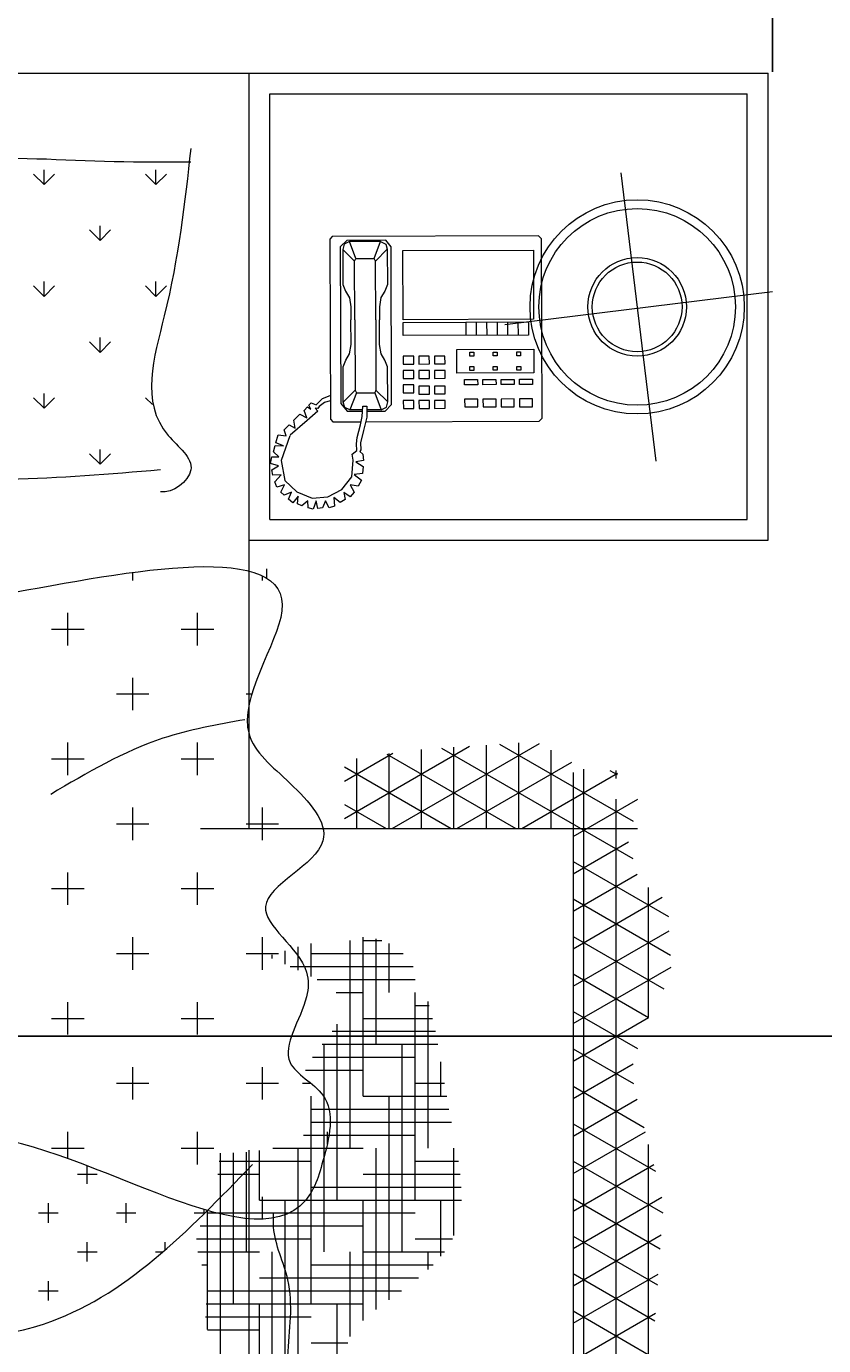
# Model space of a CAD drawing. Units: inches. Extents: x 2330 to 3943, y 1763 to 3461.
# Tile 7 of 40: x 2593 to 2634, y 2316 to 2383. Entities that reach past the tile are written whole.
import ezdxf

# ---------------------------------------------------------------- set-up
doc = ezdxf.new("R2010")
doc.units = ezdxf.units.IN
doc.layers.add('A-ANNO-DIMS', color=2, linetype='Continuous', lineweight=18)
doc.layers.add('A-FURN', color=8, linetype='Continuous', lineweight=13)
doc.styles.get("Standard").update_dxf_attribs({"font": 'arial.ttf'})
doc.dimstyles.get("Standard").update_dxf_attribs({"dimtxt": 0.18, "dimasz": 0.18, "dimexe": 0.18, "dimexo": 0.0625, "dimgap": 0.09, "dimtad": 0, "dimtih": 1, "dimtoh": 1, "dimdec": 4, "dimzin": 0, "dimdsep": 46, "dimtxsty": 'Standard', "dimcen": 0.09, "dimadec": 0, "dimazin": 0, "dimtfac": 1, "dimtdec": 4, "dimtofl": 0, "dimtmove": 0, "dimatfit": 3, "dimfxl": 1, "dimtolj": 1, "dimtzin": 0, "dimarcsym": 0})

# ---------------------------------------------------------------- blocks, each defined once
blk = doc.blocks.new('A$C200C7901')
for p, q in [((0.5, 2.3334), (2, 2.3334)), ((2, 2.3334), (2.5, 2.3334)), ((2, 1.6055), (2, 2.3334)), ((2.5, 1.8834), (2.5, 2.3334)), ((2, 1.8834), (2.5, 1.8834)), ((2.0171, 1.8467), (2.0171, 1.8556)), ((2.0171, 1.8467), (2.0171, 1.8556)), ((2.0129, 1.8445), (2.0129, 1.849)), ((2.0129, 1.8445), (2.0129, 1.849)), ((1.9972, 1.7352), (2.0027, 1.7352)), ((1.9972, 1.7352), (2.0027, 1.7352)), ((2, 1.6963), (2, 1.7248)), ((2, 1.6963), (2, 1.7248)), ((2.3121, 1.6596), (2.3121, 0.0201)), ((1.9533, 1.6055), (2.3741, 1.6055)), ((1.9533, 1.6055), (2.3741, 1.6055)), ((2, 0.2957), (2, 1.2957)), ((2.0224, 0.9977), (2.0224, 1.1977)), ((2.0224, 0.9977), (2.0224, 1.1977))]:
    blk.add_line(p, q)
at = {"linetype": 'ByBlock'}
for p, q in [((2.02, 2.3134), (2.48, 2.3134)), ((2.02, 1.9034), (2.02, 2.3134)), ((2.48, 1.9034), (2.48, 2.3134)), ((1.8025, 2.2259), (1.8025, 2.2402)), ((1.8025, 2.2259), (1.8025, 2.2402)), ((1.9103, 2.2259), (1.9103, 2.2402)), ((1.9103, 2.2259), (1.9103, 2.2402)), ((2.3581, 2.2373), (2.3919, 1.9595)), ((1.8025, 2.2259), (1.7924, 2.236)), ((1.8025, 2.2259), (1.7924, 2.236)), ((1.8025, 2.2259), (1.8126, 2.236)), ((1.8025, 2.2259), (1.8126, 2.236)), ((1.9103, 2.2259), (1.9002, 2.236)), ((1.9103, 2.2259), (1.9002, 2.236)), ((1.9103, 2.2259), (1.9204, 2.236)), ((1.9103, 2.2259), (1.9204, 2.236)), ((1.8564, 2.172), (1.8564, 2.1863)), ((1.8564, 2.172), (1.8564, 2.1863)), ((1.8564, 2.1721), (1.8463, 2.1822)), ((1.8564, 2.1721), (1.8463, 2.1822)), ((1.8564, 2.1721), (1.8665, 2.1822)), ((1.8564, 2.1721), (1.8665, 2.1822)), ((2.0802, 2.176), (2.0777, 2.1734)), ((2.0777, 2.1734), (2.0783, 1.9999)), ((2.2789, 2.1766), (2.0802, 2.176)), ((2.2789, 2.1766), (2.2814, 2.1741)), ((2.2814, 2.1741), (2.282, 2.0006)), ((2.0941, 2.1722), (2.0878, 2.1659)), ((2.0878, 2.1659), (2.0883, 2.015)), ((2.0915, 2.1685), (2.0903, 2.1634)), ((2.0903, 2.1634), (2.1017, 2.1521)), ((2.0903, 2.1634), (2.0904, 2.1295)), ((2.0966, 2.171), (2.0915, 2.1685)), ((2.1318, 2.1724), (2.0941, 2.1722)), ((2.1267, 2.1711), (2.0966, 2.171)), ((2.1029, 2.1547), (2.0966, 2.171)), ((2.1205, 2.1547), (2.1267, 2.1711)), ((2.1331, 2.1636), (2.1218, 2.1522)), ((2.1267, 2.1711), (2.1318, 2.1686)), ((2.1368, 2.1661), (2.1318, 2.1724)), ((2.1318, 2.1686), (2.1331, 2.1636)), ((2.1331, 2.1636), (2.1332, 2.1296)), ((2.1373, 2.014), (2.1368, 2.1661)), ((2.1481, 2.1624), (2.2739, 2.1628)), ((2.1484, 2.0957), (2.1481, 2.1624)), ((2.2739, 2.1628), (2.2741, 2.0961)), ((2.1017, 2.1521), (2.1029, 2.1547)), ((2.1019, 2.0956), (2.1017, 2.1521)), ((2.1029, 2.1547), (2.1205, 2.1547)), ((2.1218, 2.1522), (2.1205, 2.1547)), ((2.122, 2.0956), (2.1218, 2.1522)), ((1.8025, 2.1182), (1.7924, 2.1283)), ((1.8025, 2.1182), (1.7924, 2.1283)), ((1.8025, 2.1182), (1.8025, 2.1325)), ((1.8025, 2.1182), (1.8025, 2.1325)), ((1.8025, 2.1182), (1.8126, 2.1283)), ((1.8025, 2.1182), (1.8126, 2.1283)), ((1.9103, 2.1182), (1.9002, 2.1283)), ((1.9103, 2.1182), (1.9002, 2.1283)), ((1.9103, 2.1182), (1.9103, 2.1325)), ((1.9103, 2.1182), (1.9103, 2.1325)), ((1.9103, 2.1182), (1.9204, 2.1283)), ((1.9103, 2.1182), (1.9204, 2.1283)), ((2.0904, 2.1295), (2.093, 2.1232)), ((2.093, 2.1232), (2.0968, 2.1169)), ((2.1307, 2.1233), (2.1269, 2.117)), ((2.1332, 2.1296), (2.1307, 2.1233)), ((2.2464, 2.0911), (2.5044, 2.1228)), ((2.0968, 2.1169), (2.098, 2.1081)), ((2.1269, 2.117), (2.1257, 2.1082)), ((2.098, 2.1081), (2.0981, 2.0956)), ((2.1257, 2.1082), (2.1257, 2.0956)), ((2.0982, 2.0717), (2.0981, 2.0956)), ((2.1019, 2.0956), (2.1021, 2.0277)), ((2.122, 2.0956), (2.1222, 2.0277)), ((2.1258, 2.0718), (2.1257, 2.0956)), ((2.2741, 2.0961), (2.1484, 2.0957)), ((2.1484, 2.0932), (2.2691, 2.0936)), ((2.1484, 2.0806), (2.1484, 2.0932)), ((2.2087, 2.0934), (2.2088, 2.0808)), ((2.2188, 2.0934), (2.2188, 2.0809)), ((2.2288, 2.0935), (2.2289, 2.0809)), ((2.2389, 2.0935), (2.239, 2.0809)), ((2.249, 2.0935), (2.249, 2.081)), ((2.259, 2.0936), (2.2591, 2.081)), ((2.2691, 2.0936), (2.2691, 2.081)), ((1.8564, 2.0643), (1.8463, 2.0744)), ((1.8564, 2.0643), (1.8463, 2.0744)), ((1.8564, 2.0643), (1.8564, 2.0786)), ((1.8564, 2.0643), (1.8564, 2.0786)), ((1.8564, 2.0643), (1.8665, 2.0744)), ((1.8564, 2.0643), (1.8665, 2.0744)), ((2.0969, 2.0629), (2.0982, 2.0717)), ((2.1271, 2.063), (2.1258, 2.0718)), ((2.2691, 2.081), (2.1484, 2.0806)), ((2.0932, 2.0566), (2.0969, 2.0629)), ((2.1309, 2.0567), (2.1271, 2.063)), ((2.1586, 2.0606), (2.1485, 2.0605)), ((2.1485, 2.0605), (2.1485, 2.053)), ((2.1586, 2.053), (2.1586, 2.0606)), ((2.1636, 2.0606), (2.1636, 2.053)), ((2.1736, 2.0606), (2.1636, 2.0606)), ((2.1737, 2.0531), (2.1736, 2.0606)), ((2.1887, 2.0607), (2.1787, 2.0606)), ((2.1787, 2.0606), (2.1787, 2.0531)), ((2.1888, 2.0531), (2.1887, 2.0607)), ((2.2, 2.067), (2.2742, 2.0672)), ((2.2001, 2.0443), (2.2, 2.067)), ((2.2126, 2.0645), (2.2164, 2.0645)), ((2.2126, 2.0607), (2.2126, 2.0645)), ((2.2164, 2.0607), (2.2126, 2.0607)), ((2.2164, 2.0645), (2.2164, 2.0607)), ((2.2352, 2.0646), (2.239, 2.0646)), ((2.2352, 2.0608), (2.2352, 2.0646)), ((2.239, 2.0608), (2.2352, 2.0608)), ((2.239, 2.0646), (2.239, 2.0608)), ((2.2579, 2.0609), (2.2579, 2.0647)), ((2.2579, 2.0647), (2.2616, 2.0647)), ((2.2616, 2.0609), (2.2579, 2.0609)), ((2.2616, 2.0647), (2.2616, 2.0609)), ((2.2742, 2.0672), (2.2743, 2.0446)), ((2.0907, 2.0503), (2.0932, 2.0566)), ((2.0908, 2.0163), (2.0907, 2.0503)), ((2.1334, 2.0504), (2.1309, 2.0567)), ((2.1336, 2.0165), (2.1334, 2.0504)), ((2.1485, 2.053), (2.1586, 2.053)), ((2.1485, 2.0467), (2.1486, 2.0391)), ((2.1586, 2.0467), (2.1485, 2.0467)), ((2.1586, 2.0392), (2.1586, 2.0467)), ((2.1636, 2.053), (2.1737, 2.0531)), ((2.1737, 2.0468), (2.1636, 2.0467)), ((2.1636, 2.0467), (2.1637, 2.0392)), ((2.1737, 2.0392), (2.1737, 2.0468)), ((2.1787, 2.0531), (2.1888, 2.0531)), ((2.1787, 2.0468), (2.1787, 2.0392)), ((2.1888, 2.0468), (2.1787, 2.0468)), ((2.1888, 2.0393), (2.1888, 2.0468)), ((2.2126, 2.0507), (2.2164, 2.0507)), ((2.2127, 2.0469), (2.2126, 2.0507)), ((2.2164, 2.0469), (2.2127, 2.0469)), ((2.2164, 2.0507), (2.2164, 2.0469)), ((2.2353, 2.0508), (2.2391, 2.0508)), ((2.2353, 2.047), (2.2353, 2.0508)), ((2.2391, 2.047), (2.2353, 2.047)), ((2.2391, 2.0508), (2.2391, 2.047)), ((2.2579, 2.0508), (2.2617, 2.0508)), ((2.2579, 2.0471), (2.2579, 2.0508)), ((2.2617, 2.0471), (2.2579, 2.0471)), ((2.2617, 2.0508), (2.2617, 2.0471)), ((2.1486, 2.0391), (2.1586, 2.0392)), ((2.1637, 2.0392), (2.1737, 2.0392)), ((2.1787, 2.0392), (2.1888, 2.0393)), ((2.2743, 2.0446), (2.2001, 2.0443)), ((2.2077, 2.0331), (2.2077, 2.0381)), ((2.2077, 2.0381), (2.2202, 2.0381)), ((2.2202, 2.0381), (2.2203, 2.0331)), ((2.2253, 2.0381), (2.2378, 2.0382)), ((2.2253, 2.0331), (2.2253, 2.0381)), ((2.2378, 2.0382), (2.2379, 2.0332)), ((2.2429, 2.0332), (2.2429, 2.0382)), ((2.2429, 2.0382), (2.2554, 2.0382)), ((2.2554, 2.0382), (2.2555, 2.0332)), ((2.2605, 2.0332), (2.2605, 2.0383)), ((2.2605, 2.0383), (2.273, 2.0383)), ((2.273, 2.0383), (2.2731, 2.0333)), ((1.8025, 2.0104), (1.8025, 2.0247)), ((1.8025, 2.0104), (1.8025, 2.0247)), ((2.0707, 2.0197), (2.0782, 2.0226)), ((2.0908, 2.0163), (2.1021, 2.0277)), ((2.1034, 2.0252), (2.0971, 2.0088)), ((2.1021, 2.0277), (2.1034, 2.0252)), ((2.1034, 2.0252), (2.121, 2.0252)), ((2.1222, 2.0277), (2.121, 2.0252)), ((2.121, 2.0252), (2.1273, 2.0089)), ((2.1336, 2.0165), (2.1222, 2.0277)), ((2.1586, 2.0329), (2.1486, 2.0329)), ((2.1486, 2.0329), (2.1486, 2.0253)), ((2.1486, 2.0253), (2.1587, 2.0253)), ((2.1587, 2.0253), (2.1586, 2.0329)), ((2.1637, 2.0317), (2.1637, 2.0241)), ((2.1737, 2.0317), (2.1637, 2.0317)), ((2.1637, 2.0241), (2.1738, 2.0241)), ((2.1738, 2.0241), (2.1737, 2.0317)), ((2.1788, 2.0317), (2.1788, 2.0242)), ((2.1888, 2.0317), (2.1788, 2.0317)), ((2.1788, 2.0242), (2.1889, 2.0242)), ((2.1889, 2.0242), (2.1888, 2.0317)), ((2.2203, 2.0331), (2.2077, 2.0331)), ((2.2379, 2.0332), (2.2253, 2.0331)), ((2.2555, 2.0332), (2.2429, 2.0332)), ((2.2731, 2.0333), (2.2605, 2.0332)), ((1.8025, 2.0104), (1.7924, 2.0205)), ((1.8025, 2.0104), (1.7924, 2.0205)), ((1.8025, 2.0104), (1.8126, 2.0205)), ((1.8025, 2.0104), (1.8126, 2.0205)), ((1.9068, 2.0139), (1.9002, 2.0205)), ((1.9068, 2.0139), (1.9002, 2.0205)), ((2.053, 2.0084), (2.0563, 2.0119)), ((2.0557, 2.0011), (2.053, 2.0084)), ((2.0563, 2.0119), (2.0594, 2.0095)), ((2.0576, 2.0133), (2.0598, 2.0155)), ((2.0594, 2.0095), (2.0576, 2.0133)), ((2.0598, 2.0155), (2.0645, 2.0137)), ((2.0663, 2.0102), (2.0636, 2.0104)), ((2.0636, 2.0104), (2.0663, 2.0077)), ((2.0645, 2.0137), (2.0671, 2.0162)), ((2.0676, 2.012), (2.0663, 2.0102)), ((2.0671, 2.0162), (2.0707, 2.0197)), ((2.0727, 2.016), (2.0676, 2.012)), ((2.0782, 2.0175), (2.0727, 2.016)), ((2.0883, 2.015), (2.0946, 2.0075)), ((2.0921, 2.0113), (2.0908, 2.0163)), ((2.0971, 2.0088), (2.0921, 2.0113)), ((2.1094, 2.0088), (2.0971, 2.0088)), ((2.109, 2.0025), (2.1097, 2.0126)), ((2.1097, 2.0126), (2.1135, 2.0126)), ((2.1135, 2.0126), (2.1133, 2.0018)), ((2.1273, 2.0089), (2.1134, 2.0088)), ((2.1273, 2.0089), (2.1323, 2.0114)), ((2.1311, 2.0077), (2.1373, 2.014)), ((2.1323, 2.0114), (2.1336, 2.0165)), ((2.1587, 2.0178), (2.1486, 2.0178)), ((2.1486, 2.0178), (2.1487, 2.0102)), ((2.1487, 2.0102), (2.1587, 2.0103)), ((2.1587, 2.0103), (2.1587, 2.0178)), ((2.1738, 2.0179), (2.1637, 2.0178)), ((2.1637, 2.0178), (2.1638, 2.0103)), ((2.1638, 2.0103), (2.1738, 2.0103)), ((2.1738, 2.0103), (2.1738, 2.0179)), ((2.1788, 2.0179), (2.1788, 2.0103)), ((2.1889, 2.0179), (2.1788, 2.0179)), ((2.1788, 2.0103), (2.1889, 2.0104)), ((2.1889, 2.0104), (2.1889, 2.0179)), ((2.2203, 2.0193), (2.2077, 2.0192)), ((2.2077, 2.0192), (2.2078, 2.0117)), ((2.2078, 2.0117), (2.2203, 2.0117)), ((2.2203, 2.0117), (2.2203, 2.0193)), ((2.2379, 2.0193), (2.2253, 2.0193)), ((2.2253, 2.0193), (2.2254, 2.0117)), ((2.2254, 2.0117), (2.2379, 2.0118)), ((2.2379, 2.0118), (2.2379, 2.0193)), ((2.2555, 2.0194), (2.2429, 2.0193)), ((2.2429, 2.0193), (2.243, 2.0118)), ((2.243, 2.0118), (2.2555, 2.0118)), ((2.2555, 2.0118), (2.2555, 2.0194)), ((2.2605, 2.0194), (2.2606, 2.0119)), ((2.2731, 2.0194), (2.2605, 2.0194)), ((2.2606, 2.0119), (2.2731, 2.0119)), ((2.2731, 2.0119), (2.2731, 2.0194)), ((2.0561, 1.9986), (2.0396, 1.9844)), ((2.0431, 1.999), (2.0488, 2.0046)), ((2.0444, 1.9911), (2.0431, 1.999)), ((2.0488, 2.0046), (2.0557, 2.0011)), ((2.0663, 2.0077), (2.0561, 1.9986)), ((2.0783, 1.9999), (2.0808, 1.9974)), ((2.0808, 1.9974), (2.1079, 1.9975)), ((2.0946, 2.0075), (2.1093, 2.0076)), ((2.1072, 1.9944), (2.109, 2.0025)), ((2.1133, 2.0018), (2.1103, 1.989)), ((2.1123, 1.9975), (2.2795, 1.9981)), ((2.1134, 2.0076), (2.1311, 2.0077)), ((2.282, 2.0006), (2.2795, 1.9981)), ((2.0259, 1.977), (2.0281, 1.9847)), ((2.0281, 1.9847), (2.0358, 1.9839)), ((2.0393, 1.984), (2.031, 1.96)), ((2.0338, 1.9895), (2.0386, 1.9946)), ((2.0358, 1.9839), (2.0338, 1.9895)), ((2.0386, 1.9946), (2.0444, 1.9911)), ((2.1042, 1.9824), (2.1072, 1.9944)), ((2.1103, 1.989), (2.1073, 1.9771)), ((1.8564, 1.9565), (1.8564, 1.9708)), ((1.8564, 1.9565), (1.8564, 1.9708)), ((2.0234, 1.9686), (2.0251, 1.9745)), ((2.0251, 1.9745), (2.0333, 1.9743)), ((2.0333, 1.9743), (2.0259, 1.977)), ((2.1035, 1.9763), (2.1042, 1.9824)), ((2.1038, 1.9697), (2.1035, 1.9763)), ((2.1076, 1.9704), (2.1068, 1.9689)), ((2.1073, 1.9771), (2.1076, 1.9704)), ((1.8564, 1.9565), (1.8463, 1.9666)), ((1.8564, 1.9565), (1.8463, 1.9666)), ((1.8564, 1.9565), (1.8665, 1.9666)), ((1.8564, 1.9565), (1.8665, 1.9666)), ((2.0206, 1.9572), (2.0218, 1.9635)), ((2.0285, 1.9549), (2.0206, 1.9572)), ((2.0218, 1.9635), (2.0287, 1.9636)), ((2.0287, 1.9636), (2.0234, 1.9686)), ((2.031, 1.96), (2.0346, 1.9409)), ((2.099, 1.9444), (2.1002, 1.9605)), ((2.0992, 1.9663), (2.1038, 1.9697)), ((2.1002, 1.9605), (2.0992, 1.9663)), ((2.1101, 1.96), (2.1028, 1.9587)), ((2.1028, 1.9587), (2.1099, 1.9544)), ((2.1068, 1.9689), (2.1096, 1.9661)), ((2.1096, 1.9661), (2.1101, 1.96)), ((2.0219, 1.9511), (2.0285, 1.9549)), ((2.0229, 1.946), (2.0219, 1.9511)), ((2.0308, 1.9462), (2.0229, 1.946)), ((2.0247, 1.9394), (2.0308, 1.9462)), ((2.1094, 1.9475), (2.1013, 1.9467)), ((2.1013, 1.9467), (2.1084, 1.9412)), ((2.1099, 1.9544), (2.1094, 1.9475)), ((2.0268, 1.9343), (2.0247, 1.9394)), ((2.0341, 1.9366), (2.0268, 1.9343)), ((2.0306, 1.9297), (2.0341, 1.9366)), ((2.0346, 1.9409), (2.0459, 1.93)), ((2.0759, 1.925), (2.0894, 1.9322)), ((2.0894, 1.9322), (2.099, 1.9444)), ((2.1051, 1.9353), (2.0975, 1.9368)), ((2.0975, 1.9368), (2.1011, 1.9297)), ((2.1084, 1.9412), (2.1051, 1.9353)), ((2.0339, 1.9267), (2.0306, 1.9297)), ((2.041, 1.9297), (2.0339, 1.9267)), ((2.038, 1.9228), (2.041, 1.9297)), ((2.0421, 1.9193), (2.038, 1.9228)), ((2.0474, 1.9259), (2.0421, 1.9193)), ((2.0459, 1.93), (2.0607, 1.9237)), ((2.0467, 1.9183), (2.0474, 1.9259)), ((2.0566, 1.9214), (2.0508, 1.9163)), ((2.0569, 1.9145), (2.0566, 1.9214)), ((2.0607, 1.9237), (2.0759, 1.925)), ((2.0645, 1.9214), (2.0617, 1.9133)), ((2.0663, 1.914), (2.0645, 1.9214)), ((2.0736, 1.9214), (2.0706, 1.9146)), ((2.077, 1.9146), (2.0736, 1.9214)), ((2.0876, 1.9195), (2.0815, 1.9245)), ((2.0815, 1.9245), (2.0823, 1.9161)), ((2.0925, 1.9225), (2.0876, 1.9195)), ((2.0973, 1.9251), (2.0914, 1.9294)), ((2.0914, 1.9294), (2.0925, 1.9225)), ((2.1011, 1.9297), (2.0973, 1.9251)), ((2.0508, 1.9163), (2.0467, 1.9183)), ((2.0617, 1.9133), (2.0569, 1.9145)), ((2.0706, 1.9146), (2.0663, 1.914)), ((2.0823, 1.9161), (2.077, 1.9146)), ((2.02, 1.9034), (2.48, 1.9034)), ((1.8879, 1.8445), (1.8879, 1.8523)), ((1.8879, 1.8445), (1.8879, 1.8523)), ((1.8254, 1.782), (1.8254, 1.8133)), ((1.8254, 1.782), (1.8254, 1.8133)), ((1.9504, 1.782), (1.9504, 1.8133)), ((1.9504, 1.782), (1.9504, 1.8133)), ((1.8097, 1.7977), (1.841, 1.7977)), ((1.8097, 1.7977), (1.841, 1.7977)), ((1.9347, 1.7977), (1.966, 1.7977)), ((1.9347, 1.7977), (1.966, 1.7977)), ((1.8879, 1.7195), (1.8879, 1.7508)), ((1.8879, 1.7195), (1.8879, 1.7508)), ((1.8722, 1.7352), (1.9035, 1.7352)), ((1.8722, 1.7352), (1.9035, 1.7352)), ((1.8254, 1.657), (1.8254, 1.6883)), ((1.8254, 1.657), (1.8254, 1.6883)), ((1.9504, 1.657), (1.9504, 1.6883)), ((1.9504, 1.657), (1.9504, 1.6883)), ((2.0919, 1.6152), (2.2125, 1.6848)), ((2.0919, 1.6152), (2.2125, 1.6848)), ((2.0919, 1.6513), (2.1386, 1.6782)), ((2.0919, 1.6513), (2.1386, 1.6782)), ((2.1349, 1.6055), (2.1349, 1.6777)), ((2.1349, 1.6055), (2.1349, 1.6777)), ((2.1377, 1.6055), (2.2798, 1.6876)), ((2.1377, 1.6055), (2.2798, 1.6876)), ((2.1662, 1.6055), (2.1662, 1.6817)), ((2.1662, 1.6055), (2.1662, 1.6817)), ((2.1854, 1.683), (2.3697, 1.5766)), ((2.1854, 1.683), (2.3697, 1.5766)), ((2.1974, 1.6055), (2.1974, 1.6838)), ((2.1974, 1.6055), (2.1974, 1.6838)), ((2.2287, 1.6055), (2.2287, 1.6859)), ((2.2287, 1.6055), (2.2287, 1.6859)), ((2.2414, 1.6868), (2.3699, 1.6126)), ((2.2414, 1.6868), (2.3699, 1.6126)), ((2.2599, 1.6055), (2.2599, 1.688)), ((2.2599, 1.6055), (2.2599, 1.688)), ((2.2912, 1.6055), (2.2912, 1.6809)), ((2.2912, 1.6055), (2.2912, 1.6809)), ((1.8097, 1.6727), (1.841, 1.6727)), ((1.8097, 1.6727), (1.841, 1.6727)), ((1.9347, 1.6727), (1.966, 1.6727)), ((1.9347, 1.6727), (1.966, 1.6727)), ((2.1037, 1.6055), (2.1037, 1.673)), ((2.1037, 1.6055), (2.1037, 1.673)), ((2.1327, 1.6773), (2.2571, 1.6055)), ((2.1327, 1.6773), (2.2571, 1.6055)), ((2.2002, 1.6055), (2.3109, 1.6694)), ((2.2002, 1.6055), (2.3109, 1.6694)), ((2.0919, 1.6649), (2.1946, 1.6055)), ((2.0919, 1.6649), (2.1946, 1.6055)), ((2.2627, 1.6055), (2.3551, 1.6589)), ((2.2627, 1.6055), (2.3551, 1.6589)), ((2.3224, 0.0468), (2.3224, 1.6627)), ((2.3224, 0.0468), (2.3224, 1.6627)), ((2.3476, 1.6616), (2.3547, 1.6575)), ((2.3476, 1.6616), (2.3547, 1.6575)), ((2.3537, 1.6539), (2.3537, 1.6616)), ((2.3537, 1.6539), (2.3537, 1.6616)), ((2.0919, 1.6288), (2.1321, 1.6055)), ((2.0919, 1.6288), (2.1321, 1.6055)), ((2.3121, 1.598), (2.3745, 1.634)), ((2.3121, 1.598), (2.3745, 1.634)), ((2.3537, 0.0056), (2.3537, 1.634)), ((2.3537, 0.0056), (2.3537, 1.634)), ((1.8879, 1.5945), (1.8879, 1.6258)), ((1.8879, 1.5945), (1.8879, 1.6258)), ((2.0129, 1.5945), (2.0129, 1.6258)), ((2.0129, 1.5945), (2.0129, 1.6258)), ((1.8722, 1.6102), (1.9035, 1.6102)), ((1.8722, 1.6102), (1.9035, 1.6102)), ((1.9972, 1.6102), (2.0285, 1.6102)), ((1.9972, 1.6102), (2.0285, 1.6102)), ((2.3121, 1.5619), (2.3654, 1.5926)), ((2.3121, 1.5619), (2.3654, 1.5926)), ((1.8254, 1.532), (1.8254, 1.5633)), ((1.8254, 1.532), (1.8254, 1.5633)), ((1.9504, 1.532), (1.9504, 1.5633)), ((1.9504, 1.532), (1.9504, 1.5633)), ((2.3121, 1.5738), (2.404, 1.5208)), ((2.3121, 1.5738), (2.404, 1.5208)), ((2.3121, 1.5258), (2.3739, 1.5615)), ((2.3121, 1.5258), (2.3739, 1.5615)), ((1.8097, 1.5477), (1.841, 1.5477)), ((1.8097, 1.5477), (1.841, 1.5477)), ((1.9347, 1.5477), (1.966, 1.5477)), ((1.9347, 1.5477), (1.966, 1.5477)), ((2.3121, 1.4897), (2.3979, 1.5393)), ((2.3121, 1.4897), (2.3979, 1.5393)), ((2.3849, 1.4236), (2.3849, 1.5486)), ((2.3849, 1.4236), (2.3849, 1.5486)), ((2.3121, 1.5377), (2.406, 1.4835)), ((2.3121, 1.5377), (2.406, 1.4835)), ((1.8879, 1.4695), (1.8879, 1.5008)), ((1.8879, 1.4695), (1.8879, 1.5008)), ((2.0129, 1.4695), (2.0129, 1.5008)), ((2.0129, 1.4695), (2.0129, 1.5008)), ((2.1099, 1.3477), (2.1099, 1.5009)), ((2.1099, 1.3477), (2.1099, 1.5009)), ((2.3121, 1.4537), (2.4047, 1.5071)), ((2.3121, 1.4537), (2.4047, 1.5071)), ((2.3121, 1.5016), (2.3997, 1.4511)), ((2.3121, 1.5016), (2.3997, 1.4511)), ((2.0349, 1.4748), (2.0349, 1.4879)), ((2.0349, 1.4748), (2.0349, 1.4879)), ((2.0474, 1.4691), (2.0474, 1.4915)), ((2.0474, 1.4691), (2.0474, 1.4915)), ((2.0599, 1.4631), (2.0599, 1.4948)), ((2.0599, 1.4631), (2.0599, 1.4948)), ((2.0974, 1.2977), (2.0974, 1.4977)), ((2.0974, 1.2977), (2.0974, 1.4977)), ((2.1099, 1.4977), (2.1279, 1.4977)), ((2.1099, 1.4977), (2.1279, 1.4977)), ((2.1224, 1.3977), (2.1224, 1.4992)), ((2.1224, 1.3977), (2.1224, 1.4992)), ((2.1349, 1.4477), (2.1349, 1.4949)), ((2.1349, 1.4477), (2.1349, 1.4949)), ((1.8722, 1.4852), (1.9035, 1.4852)), ((1.8722, 1.4852), (1.9035, 1.4852)), ((1.9972, 1.4852), (2.0285, 1.4852)), ((1.9972, 1.4852), (2.0285, 1.4852)), ((2.0224, 1.4805), (2.0224, 1.4839)), ((2.0224, 1.4805), (2.0224, 1.4839)), ((2.0599, 1.4852), (2.1484, 1.4852)), ((2.0599, 1.4852), (2.1484, 1.4852)), ((2.0397, 1.4727), (2.1581, 1.4727)), ((2.0397, 1.4727), (2.1581, 1.4727)), ((2.3121, 1.4176), (2.4067, 1.4721)), ((2.3121, 1.4176), (2.4067, 1.4721)), ((2.3121, 1.4655), (2.3849, 1.4235)), ((2.3121, 1.4655), (2.3849, 1.4235)), ((2.0656, 1.4602), (2.1599, 1.4602)), ((2.0656, 1.4602), (2.1599, 1.4602)), ((1.8254, 1.407), (1.8254, 1.4383)), ((1.8254, 1.407), (1.8254, 1.4383)), ((1.9504, 1.407), (1.9504, 1.4383)), ((1.9504, 1.407), (1.9504, 1.4383)), ((2.084, 1.4477), (2.1099, 1.4477)), ((2.084, 1.4477), (2.1099, 1.4477)), ((2.0849, 1.4468), (2.0849, 1.4477)), ((2.0849, 1.4468), (2.0849, 1.4477)), ((2.1599, 1.2477), (2.1599, 1.4477)), ((2.1599, 1.2477), (2.1599, 1.4477)), ((2.1724, 1.2977), (2.1724, 1.439)), ((2.1724, 1.2977), (2.1724, 1.439)), ((2.1599, 1.4352), (2.1735, 1.4352)), ((2.1599, 1.4352), (2.1735, 1.4352)), ((2.3121, 1.4294), (2.3741, 1.3937)), ((2.3121, 1.4294), (2.3741, 1.3937)), ((2.3121, 1.3815), (2.3848, 1.4235)), ((2.3121, 1.3815), (2.3848, 1.4235)), ((1.8097, 1.4227), (1.841, 1.4227)), ((1.8097, 1.4227), (1.841, 1.4227)), ((1.9347, 1.4227), (1.966, 1.4227)), ((1.9347, 1.4227), (1.966, 1.4227)), ((2.0849, 1.2477), (2.0849, 1.4171)), ((2.0849, 1.2477), (2.0849, 1.4171)), ((2.1099, 1.4227), (2.1767, 1.4227)), ((2.1099, 1.4227), (2.1767, 1.4227)), ((2.08, 1.4102), (2.1795, 1.4102)), ((2.08, 1.4102), (2.1795, 1.4102)), ((2.0703, 1.3977), (2.1819, 1.3977)), ((2.0703, 1.3977), (2.1819, 1.3977)), ((2.0724, 1.1977), (2.0724, 1.3977)), ((2.0724, 1.1977), (2.0724, 1.3977)), ((2.1474, 1.1977), (2.1474, 1.3977)), ((2.1474, 1.1977), (2.1474, 1.3977)), ((2.3121, 1.3934), (2.3703, 1.3598)), ((2.3121, 1.3934), (2.3703, 1.3598)), ((1.8879, 1.3445), (1.8879, 1.3758)), ((1.8879, 1.3445), (1.8879, 1.3758)), ((2.0129, 1.3445), (2.0129, 1.3758)), ((2.0129, 1.3445), (2.0129, 1.3758)), ((2.0545, 1.3727), (2.1099, 1.3727)), ((2.0545, 1.3727), (2.1099, 1.3727)), ((2.0612, 1.3852), (2.1599, 1.3852)), ((2.0612, 1.3852), (2.1599, 1.3852)), ((2.1849, 1.3477), (2.1849, 1.3808)), ((2.1849, 1.3477), (2.1849, 1.3808)), ((2.3121, 1.3454), (2.37, 1.3788)), ((2.3121, 1.3454), (2.37, 1.3788)), ((1.8722, 1.3602), (1.9035, 1.3602)), ((1.8722, 1.3602), (1.9035, 1.3602)), ((1.9972, 1.3602), (2.0285, 1.3602)), ((1.9972, 1.3602), (2.0285, 1.3602)), ((2.0515, 1.3602), (2.0599, 1.3602)), ((2.0515, 1.3602), (2.0599, 1.3602)), ((2.1599, 1.3602), (2.1883, 1.3602)), ((2.1599, 1.3602), (2.1883, 1.3602)), ((2.0599, 1.1477), (2.0599, 1.3477)), ((2.0599, 1.1477), (2.0599, 1.3477)), ((2.1099, 1.3477), (2.1904, 1.3477)), ((2.1099, 1.3477), (2.1904, 1.3477)), ((2.1349, 1.1515), (2.1349, 1.3477)), ((2.1349, 1.1515), (2.1349, 1.3477)), ((2.3121, 1.3573), (2.3808, 1.3176)), ((2.3121, 1.3573), (2.3808, 1.3176)), ((2.0599, 1.3352), (2.1926, 1.3352)), ((2.0599, 1.3352), (2.1926, 1.3352)), ((2.3121, 1.3093), (2.374, 1.345)), ((2.3121, 1.3093), (2.374, 1.345)), ((2.0594, 1.3227), (2.195, 1.3227)), ((2.0594, 1.3227), (2.195, 1.3227)), ((1.8254, 1.2876), (1.8254, 1.3133)), ((1.8254, 1.2876), (1.8254, 1.3133)), ((1.9504, 1.282), (1.9504, 1.3133)), ((1.9504, 1.282), (1.9504, 1.3133)), ((2.0524, 1.3102), (2.1599, 1.3102)), ((2.0524, 1.3102), (2.1599, 1.3102)), ((2.0754, 1.3017), (2.0754, 1.3133)), ((2.0754, 1.3017), (2.0754, 1.3133)), ((2.3121, 1.3212), (2.3914, 1.2754)), ((2.3121, 1.3212), (2.3914, 1.2754)), ((2.3121, 1.2732), (2.3819, 1.3135)), ((2.3121, 1.2732), (2.3819, 1.3135)), ((1.8097, 1.2977), (1.841, 1.2977)), ((1.8097, 1.2977), (1.841, 1.2977)), ((1.9347, 1.2977), (1.966, 1.2977)), ((1.9347, 1.2977), (1.966, 1.2977)), ((2.023, 1.2977), (2.1099, 1.2977)), ((2.023, 1.2977), (2.1099, 1.2977)), ((2.0474, 1.0977), (2.0474, 1.2977)), ((2.0474, 1.0977), (2.0474, 1.2977)), ((2.0597, 1.2977), (2.0744, 1.2977)), ((2.0597, 1.2977), (2.0744, 1.2977)), ((2.1224, 1.1421), (2.1224, 1.2977)), ((2.1224, 1.1421), (2.1224, 1.2977)), ((2.1974, 1.2135), (2.1974, 1.2977)), ((2.1974, 1.2135), (2.1974, 1.2977)), ((2.3849, 1.0607), (2.3849, 1.3013)), ((2.3849, 1.0607), (2.3849, 1.3013)), ((1.9711, 1.2852), (2.0599, 1.2852)), ((1.9711, 1.2852), (2.0599, 1.2852)), ((1.9724, 1.0977), (1.9724, 1.2927)), ((1.9724, 1.0977), (1.9724, 1.2927)), ((1.9849, 1.1477), (1.9849, 1.293)), ((1.9849, 1.1477), (1.9849, 1.293)), ((1.9974, 1.1977), (1.9974, 1.2939)), ((1.9974, 1.1977), (1.9974, 1.2939)), ((2.0099, 1.2477), (2.0099, 1.2953)), ((2.0099, 1.2477), (2.0099, 1.2953)), ((2.1599, 1.2852), (2.2018, 1.2852)), ((2.1599, 1.2852), (2.2018, 1.2852)), ((2.3121, 1.2851), (2.3985, 1.2352)), ((2.3121, 1.2851), (2.3985, 1.2352)), ((1.8347, 1.2727), (1.8535, 1.2727)), ((1.8347, 1.2727), (1.8535, 1.2727)), ((1.8441, 1.2633), (1.8441, 1.2806)), ((1.8441, 1.2633), (1.8441, 1.2806)), ((1.97, 1.2727), (2.0099, 1.2727)), ((1.97, 1.2727), (2.0099, 1.2727)), ((2.1099, 1.2727), (2.2034, 1.2727)), ((2.1099, 1.2727), (2.2034, 1.2727)), ((2.3121, 1.2371), (2.3898, 1.282)), ((2.3121, 1.2371), (2.3898, 1.282)), ((2.0599, 1.2602), (2.2044, 1.2602)), ((2.0599, 1.2602), (2.2044, 1.2602)), ((2.0099, 1.2477), (2.2045, 1.2477)), ((2.0099, 1.2477), (2.2045, 1.2477)), ((2.0129, 1.2293), (2.0129, 1.2508)), ((2.0129, 1.2293), (2.0129, 1.2508)), ((2.0349, 1.0477), (2.0349, 1.2477)), ((2.0349, 1.0477), (2.0349, 1.2477)), ((2.1099, 1.1315), (2.1099, 1.2477)), ((2.1099, 1.1315), (2.1099, 1.2477)), ((2.1849, 1.1935), (2.1849, 1.2477)), ((2.1849, 1.1935), (2.1849, 1.2477)), ((2.3121, 1.2011), (2.3976, 1.2504)), ((2.3121, 1.2011), (2.3976, 1.2504)), ((2.3121, 1.249), (2.396, 1.2006)), ((2.3121, 1.249), (2.396, 1.2006)), ((1.7972, 1.2352), (1.816, 1.2352)), ((1.7972, 1.2352), (1.816, 1.2352)), ((1.8066, 1.2258), (1.8066, 1.2445)), ((1.8066, 1.2258), (1.8066, 1.2445)), ((1.8722, 1.2352), (1.891, 1.2352)), ((1.8722, 1.2352), (1.891, 1.2352)), ((1.8816, 1.2258), (1.8816, 1.2445)), ((1.8816, 1.2258), (1.8816, 1.2445)), ((1.9472, 1.2352), (1.9574, 1.2352)), ((1.9472, 1.2352), (1.9574, 1.2352)), ((1.9566, 1.2344), (1.9566, 1.2385)), ((1.9566, 1.2344), (1.9566, 1.2385)), ((1.9599, 1.1228), (1.9599, 1.2373)), ((1.9599, 1.1228), (1.9599, 1.2373)), ((1.9599, 1.2352), (2.1599, 1.2352)), ((1.9599, 1.2352), (2.1599, 1.2352)), ((2, 1.2352), (2.0285, 1.2352)), ((2, 1.2352), (2.0285, 1.2352)), ((1.953, 1.2227), (2.1099, 1.2227)), ((1.953, 1.2227), (2.1099, 1.2227)), ((1.9495, 1.2102), (2.0599, 1.2102)), ((1.9495, 1.2102), (2.0599, 1.2102)), ((2.1599, 1.2102), (2.1959, 1.2102)), ((2.1599, 1.2102), (2.1959, 1.2102)), ((2.3121, 1.165), (2.397, 1.214)), ((2.3121, 1.165), (2.397, 1.214)), ((2.3121, 1.2129), (2.3935, 1.166)), ((2.3121, 1.2129), (2.3935, 1.166)), ((1.8347, 1.1977), (1.8535, 1.1977)), ((1.8347, 1.1977), (1.8535, 1.1977)), ((1.8441, 1.1883), (1.8441, 1.207)), ((1.8441, 1.1883), (1.8441, 1.207)), ((1.9097, 1.1977), (1.917, 1.1977)), ((1.9097, 1.1977), (1.917, 1.1977)), ((1.9191, 1.1995), (1.9191, 1.207)), ((1.9191, 1.1995), (1.9191, 1.207)), ((1.9506, 1.1977), (2.0099, 1.1977)), ((1.9506, 1.1977), (2.0099, 1.1977)), ((2.0974, 1.1161), (2.0974, 1.1977)), ((2.0974, 1.1161), (2.0974, 1.1977)), ((2.1099, 1.1977), (2.1882, 1.1977)), ((2.1099, 1.1977), (2.1882, 1.1977)), ((2.1724, 1.1807), (2.1724, 1.1977)), ((2.1724, 1.1807), (2.1724, 1.1977)), ((1.9545, 1.1852), (1.9599, 1.1852)), ((1.9545, 1.1852), (1.9599, 1.1852)), ((2.0599, 1.1852), (2.1772, 1.1852)), ((2.0599, 1.1852), (2.1772, 1.1852)), ((1.8066, 1.1508), (1.8066, 1.1695)), ((1.8066, 1.1508), (1.8066, 1.1695)), ((2.0099, 1.1727), (2.1631, 1.1727)), ((2.0099, 1.1727), (2.1631, 1.1727)), ((2.3121, 1.1768), (2.3909, 1.1314)), ((2.3121, 1.1768), (2.3909, 1.1314)), ((2.3121, 1.1289), (2.3942, 1.1763)), ((2.3121, 1.1289), (2.3942, 1.1763)), ((1.7972, 1.1602), (1.816, 1.1602)), ((1.7972, 1.1602), (1.816, 1.1602)), ((1.9599, 1.1602), (2.1468, 1.1602)), ((1.9599, 1.1602), (2.1468, 1.1602)), ((1.9585, 1.1477), (2.1099, 1.1477)), ((1.9585, 1.1477), (2.1099, 1.1477)), ((2.0099, 0.9477), (2.0099, 1.1477)), ((2.0099, 0.9477), (2.0099, 1.1477)), ((2.0849, 0.9477), (2.0849, 1.1477)), ((2.0849, 0.9477), (2.0849, 1.1477)), ((1.9581, 1.1352), (2.0599, 1.1352)), ((1.9581, 1.1352), (2.0599, 1.1352)), ((2.3121, 1.1408), (2.3884, 1.0967)), ((2.3121, 1.1408), (2.3884, 1.0967)), ((2.3121, 1.0928), (2.3915, 1.1386)), ((2.3121, 1.0928), (2.3915, 1.1386)), ((1.9599, 1.1227), (2.0099, 1.1227)), ((1.9599, 1.1227), (2.0099, 1.1227)), ((2.0599, 1.1102), (2.0951, 1.1102)), ((2.0599, 1.1102), (2.0951, 1.1102))]:
    blk.add_line(p, q, dxfattribs=at)
for radius in [0.1032, 0.0947, 0.0475, 0.0432]:
    blk.add_circle((2.3739, 2.1081), radius, dxfattribs=at)
for points, knots in [([(1.9146, 1.951), (1.8174, 1.9428), (1.6601, 1.9297), (1.4574, 1.9942), (1.3549, 1.9462), (1.2593, 1.9563), (1.314, 2.0834), (1.3193, 2.1569), (1.2853, 2.2393), (1.4031, 2.2724), (1.4987, 2.2256), (1.6304, 2.2459), (1.7519, 2.2548), (1.8574, 2.2473), (1.9254, 2.2478), (1.9438, 2.2479)], [0, 0, 0, 0, 292.165466, 473.33038, 601.631673, 624.236147, 735.870502, 858.452188, 896.317728, 962.783971, 1127.3494, 1235.376134, 1347.110578, 1495.806953, 1551.11062, 1551.11062, 1551.11062, 1551.11062]), ([(1.9438, 2.2608), (1.9381, 2.2086), (1.9282, 2.1195), (1.8897, 2.0022), (1.9591, 1.9538), (1.9264, 1.9278), (1.9146, 1.93)], [0, 0, 0, 0, 163.411291, 278.570782, 318.445997, 354.484131, 354.484131, 354.484131, 354.484131]), ([(0.4485, 1.7835), (0.4321, 1.7496), (0.4062, 1.6964), (0.49, 1.6713), (0.4719, 1.5969), (0.4123, 1.592), (0.4233, 1.5337), (0.4954, 1.5086), (0.4012, 1.4738), (0.3253, 1.4306), (0.4113, 1.3764), (0.3688, 1.3065), (0.5579, 1.2663), (0.741, 1.4533), (1.1127, 1.1109), (1.4811, 1.2478), (1.7885, 1.3492), (2.0357, 1.1637), (2.0748, 1.2974), (2.0876, 1.349), (2.0192, 1.3805), (2.0564, 1.4298), (2.0588, 1.4846), (1.9759, 1.5349), (2.1004, 1.5845), (2.0397, 1.6519), (1.971, 1.7053), (2.1104, 1.8981), (1.5946, 1.7967), (1.2448, 1.7472), (0.8129, 1.7935), (0.4953, 1.8548), (0.4582, 1.7983), (0.4485, 1.7835)], [0, 0, 0, 0, 88.420092, 139.08588, 204.302936, 239.695496, 287.801042, 327.365471, 412.960499, 463.626286, 552.059846, 584.668336, 662.614915, 940.993281, 1309.926334, 1844.022653, 1996.276242, 2316.43048, 2341.441004, 2404.707416, 2449.463774, 2514.680778, 2538.40571, 2613.031547, 2697.13096, 2760.903931, 2822.692699, 2945.47, 3215.060018, 3725.584917, 4361.974444, 4504.671998, 4555.32777, 4555.32777, 4555.32777, 4555.32777]), ([(0.4856, 1.3429), (0.5504, 1.3182), (0.6715, 1.2721), (0.8374, 1.0498), (1.1164, 1.1183), (1.3878, 1.1816), (1.5888, 1.1102), (1.8403, 1.1127), (1.9415, 1.2178), (2.0032, 1.2819)], [0, 0, 0, 0, 205.411753, 383.654933, 772.067458, 921.644661, 1226.793228, 1388.983508, 1642.292305, 1642.292305, 1642.292305, 1642.292305])]:
    blk.add_open_spline(points, degree=3, knots=knots)
for points, knots in [([(1.996, 1.7104), (1.9692, 1.7057), (1.9025, 1.6938), (1.844, 1.6592), (1.809, 1.6385)], [0, 0, 0, 0, 81.132613, 201.738644, 201.738644, 201.738644, 201.738644]), ([(1.996, 1.7104), (1.9692, 1.7057), (1.9025, 1.6938), (1.844, 1.6592), (1.809, 1.6385)], [0, 0, 0, 0, 81.132613, 201.738644, 201.738644, 201.738644, 201.738644]), ([(0.473, 1.2954), (0.4739, 1.2781), (0.4755, 1.2477), (0.5032, 1.2084), (0.4801, 1.1701), (0.4928, 1.1255), (0.4674, 1.0912), (0.4579, 1.0351), (0.501, 0.9724), (0.4311, 0.8832), (0.4902, 0.8637), (0.4843, 0.8288), (0.4774, 0.7906), (0.4625, 0.7457), (0.459, 0.6999), (0.4816, 0.6664), (0.4748, 0.625), (0.4791, 0.5889), (0.4533, 0.5528), (0.4738, 0.5004), (0.4658, 0.4502), (0.4696, 0.3946), (0.4189, 0.3935), (0.4493, 0.3684), (0.4694, 0.3857), (0.4922, 0.3576), (0.5297, 0.3262), (0.5917, 0.3353), (0.6454, 0.3754), (0.7083, 0.3741), (0.7643, 0.3328), (0.826, 0.346), (0.925, 0.3388), (1.0353, 0.3593), (1.1561, 0.3744), (1.2477, 0.3154), (1.3302, 0.3474), (1.4086, 0.3512), (1.5217, 0.3878), (1.6362, 0.3176), (1.7682, 0.3285), (1.8402, 0.3019), (1.9071, 0.3529), (1.9647, 0.3412), (2.0795, 0.2948), (2.0472, 0.3498), (2.0343, 0.3772), (2.0435, 0.43), (2.0109, 0.5782), (2.0746, 0.4643), (2.0805, 0.584), (2.0084, 0.5979), (2.0343, 0.6846), (2.0344, 0.746), (2.0293, 0.8096), (2.0489, 0.8545), (2.0652, 0.9218), (1.9842, 0.9297), (2.0007, 1.0162), (2.0367, 1.0585), (2.0367, 1.1102), (2.0457, 1.1647), (2.0226, 1.2084), (2.0234, 1.2306), (2.0236, 1.2352)], [0, 0, 0, 0, 51.660678, 90.967412, 128.902454, 170.303599, 219.852997, 247.834962, 336.321557, 429.35469, 458.821847, 477.222321, 524.135809, 581.038434, 617.839381, 657.146115, 693.947125, 740.178081, 760.753248, 820.731705, 885.133458, 928.777044, 953.563729, 976.574207, 995.553042, 1018.563482, 1064.584401, 1147.951297, 1174.787598, 1266.851571, 1308.018447, 1377.066427, 1441.511314, 1608.245014, 1714.11869, 1792.771707, 1913.247991, 1954.931389, 2029.864445, 2259.189419, 2305.221512, 2429.507982, 2456.344283, 2543.92595, 2627.925037, 2662.96218, 2687.736879, 2719.937755, 2839.540991, 2875.47895, 2953.681041, 2993.270313, 3066.872333, 3154.395764, 3200.397042, 3248.426375, 3312.828127, 3347.881398, 3444.484026, 3481.577522, 3518.665244, 3592.267265, 3644.719162, 3658.519501, 3658.519501, 3658.519501, 3658.519501])]:
    blk.add_open_spline(points, degree=3, knots=knots, dxfattribs=at)
blk = doc.blocks.new('*D39')
at = {"layer": 'A-ANNO-DIMS', "color": 0, "lineweight": -2, "transparency": 16777216}
for p, q in [((2499.499, 2380.496), (2499.499, 2400.343)), ((2499.679, 2400.163), (2563.823, 2400.163)), ((2630.845, 2400.163), (2566.701, 2400.163)), ((2631.025, 2380.496), (2631.025, 2400.343))]:
    blk.add_line(p, q, dxfattribs=at)
at = {"layer": 'A-ANNO-DIMS', "color": 0, "transparency": 16777216}
for points in [[(2499.679, 2400.193), (2499.679, 2400.133), (2499.499, 2400.163)], [(2630.845, 2400.193), (2630.845, 2400.133), (2631.025, 2400.163)]]:
    blk.add_solid(points, dxfattribs=at)
at = {"layer": 'Defpoints', "color": 0, "transparency": 16777216}
for p in [(2631.025, 2400.163), (2499.499, 2380.434), (2631.025, 2380.434)]:
    blk.add_point(p, dxfattribs=at)
at = {"layer": 'A-ANNO-DIMS', "color": 0, "transparency": 16777216, "insert": (2565.262, 2400.163), "char_height": 0.18, "attachment_point": 5}
blk.add_mtext('\\A1;DOUBLE BED 132 TYP.', dxfattribs=at)
blk = doc.blocks.new('*D80')
at = {"layer": 'A-ANNO-DIMS', "color": 0, "lineweight": -2, "transparency": 16777216}
for p, q in [((3166.598, 2331.698), (2330.502, 2331.698)), ((2330.682, 2331.518), (2330.682, 2322.357)), ((2330.682, 2312.832), (2330.682, 2321.993)), ((3166.598, 2312.652), (2330.502, 2312.652))]:
    blk.add_line(p, q, dxfattribs=at)
at = {"layer": 'A-ANNO-DIMS', "color": 0, "transparency": 16777216}
for points in [[(2330.652, 2331.518), (2330.712, 2331.518), (2330.682, 2331.698)], [(2330.652, 2312.832), (2330.712, 2312.832), (2330.682, 2312.652)]]:
    blk.add_solid(points, dxfattribs=at)
at = {"layer": 'Defpoints', "color": 0, "transparency": 16777216}
for p in [(2330.682, 2331.698), (3166.661, 2331.698), (3166.661, 2312.652)]:
    blk.add_point(p, dxfattribs=at)
at = {"layer": 'A-ANNO-DIMS', "color": 0, "transparency": 16777216, "insert": (2330.682, 2322.175), "char_height": 0.18, "attachment_point": 5}
blk.add_mtext('\\A1;19.046', dxfattribs=at)

msp = doc.modelspace()

# ---------------------------------------------------------------- block references
at = {"layer": 'A-FURN', "xscale": 52.5181391560459, "yscale": 52.5181391560459, "zscale": 52.5181391560459}
msp.add_blockref('A$C200C7901', (2499.4987, 2257.8888), dxfattribs=at)

# ---------------------------------------------------------------- dimensions: what is measured, and where the dimension line sits
at = {"layer": 'A-ANNO-DIMS'}
dim = msp.add_linear_dim(base=(2631.0254, 2400.1629), p1=(2499.4986, 2380.4339), p2=(2631.0254, 2380.4339), text='DOUBLE BED <> TYP.', dimstyle='Standard', override={"dimdec": 0, "dimlfac": 1, "dimrnd": 0, "dimzin": 0, "dimdsep": 46, "dimlunit": 2}, dxfattribs=at)
dim.commit()
dim.dimension.update_dxf_attribs({"geometry": '*D39', "text_midpoint": (2565.262, 2400.1629)})
dim = msp.add_linear_dim(base=(2330.6824, 2331.6982), p1=(3166.6605, 2312.6524), p2=(3166.6605, 2331.6982), angle=90, dimstyle='Standard', override={"dimdec": 3, "dimlfac": 1, "dimrnd": 0, "dimzin": 0, "dimdsep": 46, "dimlunit": 2}, dxfattribs=at)
dim.commit()
dim.dimension.update_dxf_attribs({"geometry": '*D80', "text_midpoint": (2330.6824, 2322.1753)})

doc.saveas('drawing.dxf')
